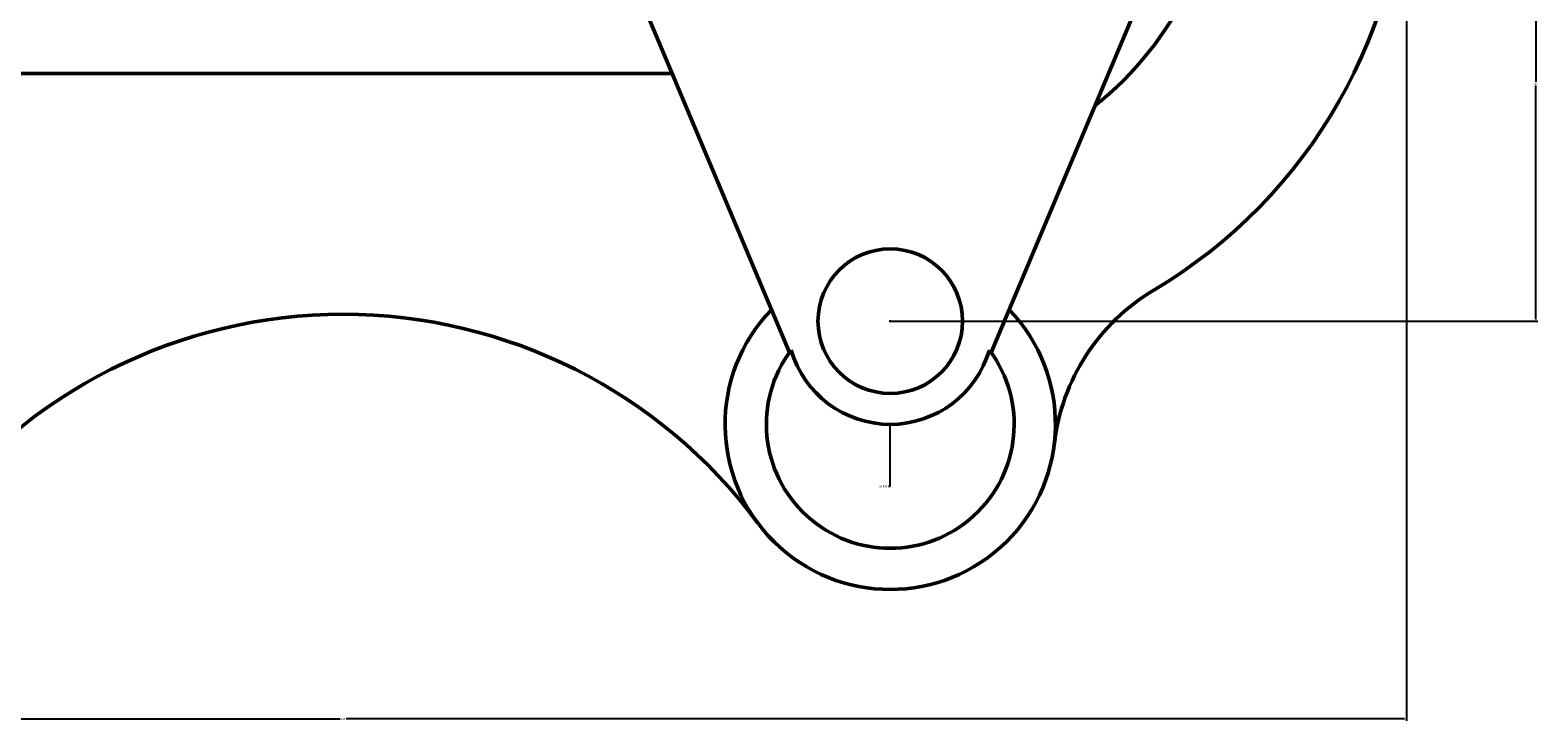
# Model space of a CAD drawing. Units: inches. Extents: x -307 to -76, y 16 to 196.
# Tile 4 of 7: x -222 to -76, y 16 to 83. Entities that reach past the tile are written whole.
import ezdxf

# ---------------------------------------------------------------- set-up
doc = ezdxf.new("R2010")
doc.units = ezdxf.units.IN
doc.header["$MEASUREMENT"] = 0
for name, color, linetype, lineweight in [('M-DIMS', 2, 'Continuous', 18), ('M-OUTL', 7, 'Continuous', 50), ('M-OUTL-LINK', 7, 'Continuous', 50)]:
    doc.layers.add(name, color=color, linetype=linetype, lineweight=lineweight)
doc.styles.get("Standard").update_dxf_attribs({"font": 'arial.ttf'})
doc.dimstyles.get("Standard").update_dxf_attribs({"dimtxt": 0.18, "dimasz": 0.18, "dimexe": 0.18, "dimexo": 0.0625, "dimgap": 0.09, "dimtad": 0, "dimtih": 1, "dimtoh": 1, "dimdec": 4, "dimzin": 0, "dimdsep": 46, "dimtxsty": 'Standard', "dimcen": 0.09, "dimadec": 0, "dimazin": 0, "dimtfac": 1, "dimtdec": 4, "dimtofl": 0, "dimtmove": 0, "dimatfit": 3, "dimfxl": 1, "dimtolj": 1, "dimtzin": 0, "dimarcsym": 0})

# ---------------------------------------------------------------- blocks, each defined once
blk = doc.blocks.new('*D2')
at = {"layer": 'Defpoints', "color": 0, "transparency": 16777216}
for p in [(-294.39, 101), (-88.39, 101), (-88.39, 16.45)]:
    blk.add_point(p, dxfattribs=at)
at = {"layer": 'M-DIMS', "color": 0, "lineweight": -2, "transparency": 16777216}
for p, q in [((-294.39, 100.94), (-294.39, 16.27)), ((-88.39, 100.94), (-88.39, 16.27)), ((-294.21, 16.45), (-191.68, 16.45)), ((-88.57, 16.45), (-191.1, 16.45))]:
    blk.add_line(p, q, dxfattribs=at)
at = {"layer": 'M-DIMS', "color": 0, "transparency": 16777216}
for points in [[(-294.21, 16.48), (-294.21, 16.42), (-294.39, 16.45)], [(-88.57, 16.48), (-88.57, 16.42), (-88.39, 16.45)]]:
    blk.add_solid(points, dxfattribs=at)
at = {"layer": 'M-DIMS', "color": 0, "transparency": 16777216, "insert": (-191.39, 16.45), "char_height": 0.18, "attachment_point": 5}
blk.add_mtext('\\A1;206', dxfattribs=at)
blk = doc.blocks.new('*D8')
at = {"layer": 'Defpoints', "color": 0, "transparency": 16777216}
for p in [(-138.39, 101), (-75.84, 101), (-138.39, 55)]:
    blk.add_point(p, dxfattribs=at)
at = {"layer": 'M-DIMS', "color": 0, "lineweight": -2, "transparency": 16777216}
for p, q in [((-138.33, 101), (-75.66, 101)), ((-75.84, 100.82), (-75.84, 78.18)), ((-75.84, 55.18), (-75.84, 77.82)), ((-138.33, 55), (-75.66, 55))]:
    blk.add_line(p, q, dxfattribs=at)
at = {"layer": 'M-DIMS', "color": 0, "transparency": 16777216}
for points in [[(-75.87, 100.82), (-75.81, 100.82), (-75.84, 101)], [(-75.87, 55.18), (-75.81, 55.18), (-75.84, 55)]]:
    blk.add_solid(points, dxfattribs=at)
at = {"layer": 'M-DIMS', "color": 0, "transparency": 16777216, "insert": (-75.84, 78), "char_height": 0.18, "attachment_point": 5}
blk.add_mtext('\\A1;46', dxfattribs=at)
blk = doc.blocks.new('*D17')
at = {"layer": 'Defpoints', "color": 0, "transparency": 16777216}
for p in [(-138.39, 55), (-138.39, 45)]:
    blk.add_point(p, dxfattribs=at)
at = {"layer": 'M-DIMS', "color": 0, "lineweight": -2, "transparency": 16777216}
for p, q in [((-138.48, 55), (-138.3, 55)), ((-138.39, 54.91), (-138.39, 55.09)), ((-138.39, 39), (-138.39, 44.82)), ((-138.57, 39), (-138.39, 39))]:
    blk.add_line(p, q, dxfattribs=at)
at = {"layer": 'M-DIMS', "color": 0, "transparency": 16777216}
blk.add_solid([(-138.42, 44.82), (-138.36, 44.82), (-138.39, 45)], dxfattribs=at)
at = {"layer": 'M-DIMS', "color": 0, "transparency": 16777216, "insert": (-139.07, 39), "char_height": 0.18, "attachment_point": 5}
blk.add_mtext('\\A1;2X R10', dxfattribs=at)

msp = doc.modelspace()

# ---------------------------------------------------------------- linework, layer by layer
at = {"layer": 'M-OUTL'}
msp.add_line((-244.39, 79), (-159.52, 79), dxfattribs=at)
for centre, radius, start, end in [((-138.39, 101), 50, 300.7178, 59.2822), ((-138.39, 101), 32, 308.26, 53.1888), ((-102.63, 40.82), 20, 120.7178, 173.3346), ((-191.39, 5.67), 50, 36.5795, 143.4205), ((-138.39, 45), 16, 136.0224, 43.9776), ((-138.39, 45), 12, 143.1301, 36.8699), ((-138.39, 101), 50, 258.7292, 259.0337), ((-138.39, 101), 50, 280.9663, 281.2708)]:
    msp.add_arc(centre, radius, start, end, dxfattribs=at)
at = {"layer": 'M-OUTL-LINK'}
for p, q in [((-148.16, 51.96), (-164.2, 90.16)), ((-128.62, 51.96), (-112.57, 90.16))]:
    msp.add_line(p, q, dxfattribs=at)
msp.add_circle((-138.39, 55), 7, dxfattribs=at)
msp.add_arc((-138.39, 55), 10, 196.2602, 343.7398, dxfattribs=at)

# ---------------------------------------------------------------- dimensions: what is measured, and where the dimension line sits
at = {"layer": 'M-DIMS'}
dim = msp.add_linear_dim(base=(-88.39, 16.45), p1=(-294.39, 101), p2=(-88.39, 101), dimstyle='Standard', override={"dimdec": 0, "dimlfac": 1, "dimrnd": 0, "dimzin": 0, "dimdsep": 46, "dimlunit": 2}, dxfattribs=at)
dim.commit()
dim.dimension.update_dxf_attribs({"geometry": '*D2', "text_midpoint": (-191.39, 16.45)})
dim = msp.add_linear_dim(base=(-75.84, 101), p1=(-138.39, 55), p2=(-138.39, 101), angle=90, dimstyle='Standard', override={"dimdec": 0, "dimlfac": 1, "dimrnd": 0, "dimzin": 0, "dimdsep": 46, "dimlunit": 2}, dxfattribs=at)
dim.commit()
dim.dimension.update_dxf_attribs({"geometry": '*D8', "text_midpoint": (-75.84, 78)})
dim = msp.add_radius_dim(center=(-138.39, 55), mpoint=(-138.39, 45), text='2X <>', dimstyle='Standard', override={"dimdec": 0, "dimlfac": 1, "dimrnd": 0, "dimzin": 0, "dimdsep": 46, "dimlunit": 2}, dxfattribs=at)
dim.commit()
dim.dimension.update_dxf_attribs({"geometry": '*D17', "text_midpoint": (-139.07, 39), "dimtype": 164})

doc.saveas('drawing.dxf')
